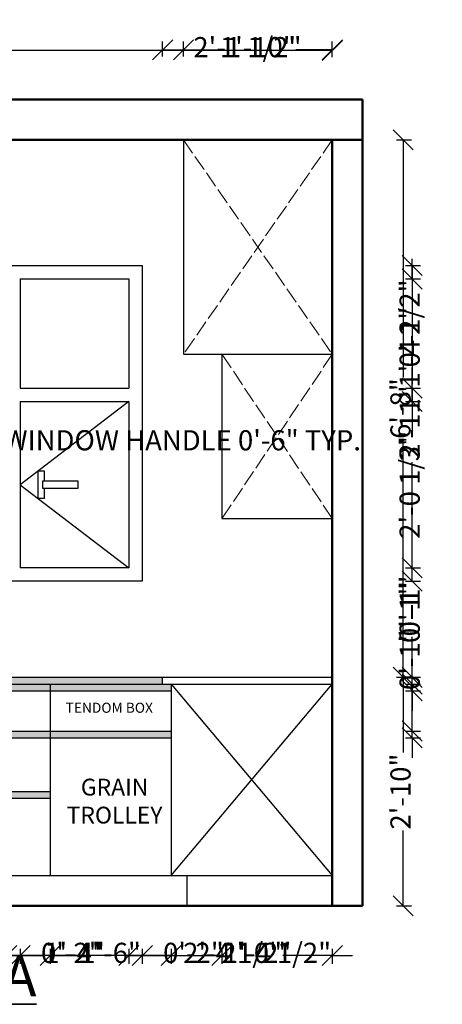
# Model space of a CAD drawing. Units: inches. Extents: x 2164 to 2316, y 625 to 771.
# Tile 2 of 2: x 2253 to 2316, y 625 to 771. Entities that reach past the tile are written whole.
import ezdxf

# ---------------------------------------------------------------- set-up
doc = ezdxf.new("R2010")
doc.units = ezdxf.units.IN
doc.linetypes.add('ACAD_ISO02W100', pattern=[15, 12, -3])
for name, color, linetype, lineweight in [('A-ANNO-DIMS', 2, 'Continuous', 18), ('A-ANNO-TEXT', 7, 'Continuous', 18), ('A-ANNO-TTLB', 7, 'Continuous', 35), ('A-FURN', 30, 'Continuous', 25), ('A-FURN-OPEN', 8, 'ACAD_ISO02W100', 13), ('A-FURN-PATT', 8, 'Continuous', 13), ('A-GLAZ', 4, 'Continuous', 25), ('A-WALL', 7, 'Continuous', 50)]:
    doc.layers.add(name, color=color, linetype=linetype, lineweight=lineweight)
doc.styles.get("Standard").update_dxf_attribs({"font": 'arial.ttf'})
doc.dimstyles.new('ISO-25', dxfattribs={"dimtxt": 3, "dimasz": 3, "dimexe": 1.25, "dimexo": 0.625, "dimtad": 0, "dimdec": 5, "dimlunit": 4, "dimtxsty": 'Standard', "dimblk": 'OBLIQUE', "dimcen": 2.5, "dimclrt": 1, "dimadec": 0, "dimazin": 0, "dimtfac": 1, "dimtdec": 5, "dimtmove": 0, "dimatfit": 3, "dimldrblk": 'OBLIQUE', "dimfxl": 1, "dimfxlon": 1, "dimfrac": 1, "dimarcsym": 0})

# ---------------------------------------------------------------- blocks, each defined once
blk = doc.blocks.new('_Oblique')
at = {"color": 0, "linetype": 'ByBlock', "lineweight": -2}
blk.add_line((-0.5, -0.5), (0.5, 0.5), dxfattribs=at)
blk = doc.blocks.new('*D4')
at = {"layer": 'A-ANNO-DIMS', "color": 0, "lineweight": -2, "transparency": 16777216}
for p, q in [((2180.45, 765.55), (2180.45, 767.8)), ((2180.45, 766.55), (2232.28, 766.55)), ((2299.95, 766.55), (2248.13, 766.55)), ((2299.95, 765.55), (2299.95, 767.8))]:
    blk.add_line(p, q, dxfattribs=at)
at = {"layer": 'Defpoints', "color": 0, "transparency": 16777216}
for p in [(2299.95, 766.55), (2180.45, 759.25), (2299.95, 759.25)]:
    blk.add_point(p, dxfattribs=at)
at = {"layer": 'A-ANNO-DIMS', "color": 0, "lineweight": -2, "transparency": 16777216, "xscale": 3, "yscale": 3, "zscale": 3, "rotation": 180}
blk.add_blockref('_Oblique', (2180.45, 766.55), dxfattribs=at)
at = {"layer": 'A-ANNO-DIMS', "color": 0, "lineweight": -2, "transparency": 16777216, "xscale": 3, "yscale": 3, "zscale": 3}
blk.add_blockref('_Oblique', (2299.95, 766.55), dxfattribs=at)
at = {"layer": 'A-ANNO-DIMS', "color": 0, "transparency": 16777216, "insert": (2240.2, 766.55), "char_height": 3, "attachment_point": 5}
blk.add_mtext('9\'-11{\\H1x;\\S1#2;}"', dxfattribs=at)
blk = doc.blocks.new('*D5')
at = {"layer": 'A-ANNO-DIMS', "color": 0, "lineweight": -2, "transparency": 16777216}
for p, q in [((2309.49, 673.25), (2311.74, 673.25)), ((2310.49, 673.25), (2310.49, 662.06)), ((2310.49, 639.25), (2310.49, 650.45)), ((2309.49, 639.25), (2311.74, 639.25))]:
    blk.add_line(p, q, dxfattribs=at)
at = {"layer": 'Defpoints', "color": 0, "transparency": 16777216}
for p in [(2299.95, 673.25), (2310.49, 673.25), (2299.95, 639.25)]:
    blk.add_point(p, dxfattribs=at)
at = {"layer": 'A-ANNO-DIMS', "color": 0, "lineweight": -2, "transparency": 16777216, "xscale": 3, "yscale": 3, "zscale": 3}
for p, rotation in [((2310.49, 673.25), 90), ((2310.49, 639.25), 270)]:
    blk.add_blockref('_Oblique', p, dxfattribs=dict(at, rotation=rotation))
at = {"layer": 'A-ANNO-DIMS', "color": 0, "transparency": 16777216, "insert": (2310.49, 656.25), "char_height": 3, "attachment_point": 5, "rotation": 90}
blk.add_mtext('2\'-10"', dxfattribs=at)
blk = doc.blocks.new('*D6')
at = {"layer": 'A-ANNO-DIMS', "color": 0, "lineweight": -2, "transparency": 16777216}
for p, q in [((2309.49, 753.25), (2311.74, 753.25)), ((2310.49, 753.25), (2310.49, 717.87)), ((2310.49, 673.25), (2310.49, 708.63)), ((2309.49, 673.25), (2311.74, 673.25))]:
    blk.add_line(p, q, dxfattribs=at)
at = {"layer": 'Defpoints', "color": 0, "transparency": 16777216}
for p in [(2299.95, 753.25), (2310.49, 753.25), (2299.95, 673.25)]:
    blk.add_point(p, dxfattribs=at)
at = {"layer": 'A-ANNO-DIMS', "color": 0, "lineweight": -2, "transparency": 16777216, "xscale": 3, "yscale": 3, "zscale": 3}
for p, rotation in [((2310.49, 753.25), 90), ((2310.49, 673.25), 270)]:
    blk.add_blockref('_Oblique', p, dxfattribs=dict(at, rotation=rotation))
at = {"layer": 'A-ANNO-DIMS', "color": 0, "transparency": 16777216, "insert": (2310.49, 713.25), "char_height": 3, "attachment_point": 5, "rotation": 90}
blk.add_mtext('6\'-8"', dxfattribs=at)
blk = doc.blocks.new('WIN-HANDLE')
blk.add_lwpolyline([(2239.92, 710.04), (2239.92, 709.04), (2240.92, 709.04), (2240.92, 710.54), (2245.92, 710.54), (2245.92, 711.54), (2240.92, 711.54), (2240.92, 713.04), (2239.92, 713.04), (2239.92, 711.04)], close=True)
blk.add_lwpolyline([(2240.92, 711.54), (2240.62, 711.54), (2240.62, 710.54), (2240.92, 710.54)])
blk = doc.blocks.new('*D8')
at = {"layer": 'A-ANNO-DIMS', "color": 0, "lineweight": -2, "transparency": 16777216}
for p, q in [((2239.92, 708.42), (2239.92, 706.89)), ((2239.92, 708.14), (2245.92, 708.14)), ((2245.92, 708.42), (2245.92, 706.89)), ((2245.92, 708.14), (2248.92, 708.14))]:
    blk.add_line(p, q, dxfattribs=at)
at = {"layer": 'Defpoints', "color": 0, "transparency": 16777216}
for p in [(2239.92, 709.04), (2245.92, 709.04), (2245.92, 708.14)]:
    blk.add_point(p, dxfattribs=at)
at = {"layer": 'A-ANNO-DIMS', "color": 0, "lineweight": -2, "transparency": 16777216, "xscale": 3, "yscale": 3, "zscale": 3, "rotation": 180}
blk.add_blockref('_Oblique', (2239.92, 708.14), dxfattribs=at)
at = {"layer": 'A-ANNO-DIMS', "color": 0, "lineweight": -2, "transparency": 16777216, "xscale": 3, "yscale": 3, "zscale": 3}
blk.add_blockref('_Oblique', (2245.92, 708.14), dxfattribs=at)
at = {"layer": 'A-ANNO-DIMS', "color": 1, "transparency": 16777216, "insert": (2277.61, 708.14), "char_height": 3, "attachment_point": 5}
blk.add_mtext('WINDOW HANDLE 0\'-6" TYP.', dxfattribs=at)
blk = doc.blocks.new('*D11')
at = {"layer": 'A-ANNO-DIMS', "color": 0, "lineweight": -2, "transparency": 16777216}
for p, q in [((2277.79, 765.65), (2277.79, 767.9)), ((2299.95, 765.65), (2299.95, 767.9)), ((2277.79, 766.65), (2283.23, 766.65)), ((2299.95, 766.65), (2294.51, 766.65))]:
    blk.add_line(p, q, dxfattribs=at)
at = {"layer": 'Defpoints', "color": 0, "transparency": 16777216}
for p in [(2299.95, 766.65), (2277.79, 753.25), (2299.95, 753.25)]:
    blk.add_point(p, dxfattribs=at)
at = {"layer": 'A-ANNO-DIMS', "color": 0, "lineweight": -2, "transparency": 16777216, "xscale": 3, "yscale": 3, "zscale": 3, "rotation": 180}
blk.add_blockref('_Oblique', (2277.79, 766.65), dxfattribs=at)
at = {"layer": 'A-ANNO-DIMS', "color": 0, "lineweight": -2, "transparency": 16777216, "xscale": 3, "yscale": 3, "zscale": 3}
blk.add_blockref('_Oblique', (2299.95, 766.65), dxfattribs=at)
at = {"layer": 'A-ANNO-DIMS', "color": 1, "transparency": 16777216, "insert": (2288.87, 766.65), "char_height": 3, "attachment_point": 5}
blk.add_mtext('1\'-10"', dxfattribs=at)
blk = doc.blocks.new('*D15')
at = {"layer": 'A-ANNO-DIMS', "color": 0, "lineweight": -2, "transparency": 16777216}
for p, q in [((2283.52, 631.85), (2280.52, 631.85)), ((2283.52, 632.85), (2283.52, 630.6)), ((2283.52, 631.85), (2283.77, 631.85)), ((2299.95, 631.85), (2299.7, 631.85)), ((2299.95, 632.85), (2299.95, 630.6)), ((2299.95, 631.85), (2302.95, 631.85))]:
    blk.add_line(p, q, dxfattribs=at)
at = {"layer": 'Defpoints', "color": 0, "transparency": 16777216}
for p in [(2283.52, 696.88), (2299.95, 696.88), (2299.95, 631.85)]:
    blk.add_point(p, dxfattribs=at)
at = {"layer": 'A-ANNO-DIMS', "color": 0, "lineweight": -2, "transparency": 16777216, "xscale": 3, "yscale": 3, "zscale": 3}
blk.add_blockref('_Oblique', (2283.52, 631.85), dxfattribs=at)
at = {"layer": 'A-ANNO-DIMS', "color": 0, "lineweight": -2, "transparency": 16777216, "xscale": 3, "yscale": 3, "zscale": 3, "rotation": 180}
blk.add_blockref('_Oblique', (2299.95, 631.85), dxfattribs=at)
at = {"layer": 'A-ANNO-DIMS', "color": 1, "transparency": 16777216, "insert": (2291.73, 631.85), "char_height": 3, "attachment_point": 5}
blk.add_mtext('1\'-4 1/2"', dxfattribs=at)
blk = doc.blocks.new('*D16')
at = {"layer": 'A-ANNO-DIMS', "color": 0, "lineweight": -2, "transparency": 16777216}
for p, q in [((2271.66, 632.85), (2271.66, 630.6)), ((2271.66, 631.85), (2277.68, 631.85)), ((2299.95, 631.85), (2293.94, 631.85)), ((2299.95, 632.85), (2299.95, 630.6))]:
    blk.add_line(p, q, dxfattribs=at)
at = {"layer": 'Defpoints', "color": 0, "transparency": 16777216}
for p in [(2299.95, 696.88), (2271.66, 687.55), (2299.95, 631.85)]:
    blk.add_point(p, dxfattribs=at)
at = {"layer": 'A-ANNO-DIMS', "color": 0, "lineweight": -2, "transparency": 16777216, "xscale": 3, "yscale": 3, "zscale": 3, "rotation": 180}
blk.add_blockref('_Oblique', (2271.66, 631.85), dxfattribs=at)
at = {"layer": 'A-ANNO-DIMS', "color": 0, "lineweight": -2, "transparency": 16777216, "xscale": 3, "yscale": 3, "zscale": 3}
blk.add_blockref('_Oblique', (2299.95, 631.85), dxfattribs=at)
at = {"layer": 'A-ANNO-DIMS', "color": 1, "transparency": 16777216, "insert": (2285.81, 631.85), "char_height": 3, "attachment_point": 5}
blk.add_mtext('2\'-4 1/2"', dxfattribs=at)
blk = doc.blocks.new('*D20')
at = {"layer": 'A-ANNO-DIMS', "color": 0, "lineweight": -2, "transparency": 16777216}
for p, q in [((2251.49, 632.85), (2251.49, 630.6)), ((2251.49, 631.85), (2253.49, 631.85)), ((2253.49, 632.85), (2253.49, 630.6)), ((2253.49, 631.85), (2256.49, 631.85))]:
    blk.add_line(p, q, dxfattribs=at)
at = {"layer": 'Defpoints', "color": 0, "transparency": 16777216}
for p in [(2251.49, 689.55), (2253.49, 689.55), (2253.49, 631.85)]:
    blk.add_point(p, dxfattribs=at)
at = {"layer": 'A-ANNO-DIMS', "color": 0, "lineweight": -2, "transparency": 16777216, "xscale": 3, "yscale": 3, "zscale": 3, "rotation": 180}
blk.add_blockref('_Oblique', (2251.49, 631.85), dxfattribs=at)
at = {"layer": 'A-ANNO-DIMS', "color": 0, "lineweight": -2, "transparency": 16777216, "xscale": 3, "yscale": 3, "zscale": 3}
blk.add_blockref('_Oblique', (2253.49, 631.85), dxfattribs=at)
at = {"layer": 'A-ANNO-DIMS', "color": 1, "transparency": 16777216, "insert": (2261.11, 631.85), "char_height": 3, "attachment_point": 5}
blk.add_mtext('0\'-2"', dxfattribs=at)
blk = doc.blocks.new('*D21')
at = {"layer": 'A-ANNO-DIMS', "color": 0, "lineweight": -2, "transparency": 16777216}
for p, q in [((2253.49, 632.85), (2253.49, 630.6)), ((2253.49, 631.85), (2257.11, 631.85)), ((2269.66, 631.85), (2266.05, 631.85)), ((2269.66, 632.85), (2269.66, 630.6))]:
    blk.add_line(p, q, dxfattribs=at)
at = {"layer": 'Defpoints', "color": 0, "transparency": 16777216}
for p in [(2253.49, 689.55), (2269.66, 689.55), (2269.66, 631.85)]:
    blk.add_point(p, dxfattribs=at)
at = {"layer": 'A-ANNO-DIMS', "color": 0, "lineweight": -2, "transparency": 16777216, "xscale": 3, "yscale": 3, "zscale": 3, "rotation": 180}
blk.add_blockref('_Oblique', (2253.49, 631.85), dxfattribs=at)
at = {"layer": 'A-ANNO-DIMS', "color": 0, "lineweight": -2, "transparency": 16777216, "xscale": 3, "yscale": 3, "zscale": 3}
blk.add_blockref('_Oblique', (2269.66, 631.85), dxfattribs=at)
at = {"layer": 'A-ANNO-DIMS', "color": 1, "transparency": 16777216, "insert": (2261.58, 631.85), "char_height": 3, "attachment_point": 5}
blk.add_mtext('1\'-4"', dxfattribs=at)
blk = doc.blocks.new('*D22')
at = {"layer": 'A-ANNO-DIMS', "color": 0, "lineweight": -2, "transparency": 16777216}
for p, q in [((2269.66, 632.85), (2269.66, 630.6)), ((2269.66, 631.85), (2271.66, 631.85)), ((2271.66, 632.85), (2271.66, 630.6)), ((2271.66, 631.85), (2274.66, 631.85))]:
    blk.add_line(p, q, dxfattribs=at)
at = {"layer": 'Defpoints', "color": 0, "transparency": 16777216}
for p in [(2269.66, 689.55), (2271.66, 687.55), (2271.66, 631.85)]:
    blk.add_point(p, dxfattribs=at)
at = {"layer": 'A-ANNO-DIMS', "color": 0, "lineweight": -2, "transparency": 16777216, "xscale": 3, "yscale": 3, "zscale": 3, "rotation": 180}
blk.add_blockref('_Oblique', (2269.66, 631.85), dxfattribs=at)
at = {"layer": 'A-ANNO-DIMS', "color": 0, "lineweight": -2, "transparency": 16777216, "xscale": 3, "yscale": 3, "zscale": 3}
blk.add_blockref('_Oblique', (2271.66, 631.85), dxfattribs=at)
at = {"layer": 'A-ANNO-DIMS', "color": 1, "transparency": 16777216, "insert": (2279.28, 631.85), "char_height": 3, "attachment_point": 5}
blk.add_mtext('0\'-2"', dxfattribs=at)
blk = doc.blocks.new('*D23')
at = {"layer": 'A-ANNO-DIMS', "color": 0, "lineweight": -2, "transparency": 16777216}
for p, q in [((2209.01, 632.85), (2209.01, 630.6)), ((2209.01, 631.85), (2232.23, 631.85)), ((2271.66, 631.85), (2248.44, 631.85)), ((2271.66, 632.85), (2271.66, 630.6))]:
    blk.add_line(p, q, dxfattribs=at)
at = {"layer": 'Defpoints', "color": 0, "transparency": 16777216}
for p in [(2209.01, 687.55), (2271.66, 687.55), (2271.66, 631.85)]:
    blk.add_point(p, dxfattribs=at)
at = {"layer": 'A-ANNO-DIMS', "color": 0, "lineweight": -2, "transparency": 16777216, "xscale": 3, "yscale": 3, "zscale": 3, "rotation": 180}
blk.add_blockref('_Oblique', (2209.01, 631.85), dxfattribs=at)
at = {"layer": 'A-ANNO-DIMS', "color": 0, "lineweight": -2, "transparency": 16777216, "xscale": 3, "yscale": 3, "zscale": 3}
blk.add_blockref('_Oblique', (2271.66, 631.85), dxfattribs=at)
at = {"layer": 'A-ANNO-DIMS', "color": 1, "transparency": 16777216, "insert": (2240.33, 631.85), "char_height": 3, "attachment_point": 5}
blk.add_mtext('5\'-2 1/2"', dxfattribs=at)
blk = doc.blocks.new('*D24')
at = {"layer": 'A-ANNO-DIMS', "color": 0, "lineweight": -2, "transparency": 16777216}
for p, q in [((2310.85, 734.54), (2313.1, 734.54)), ((2311.85, 734.54), (2311.85, 716.82)), ((2311.85, 687.55), (2311.85, 705.27)), ((2310.85, 687.55), (2313.1, 687.55))]:
    blk.add_line(p, q, dxfattribs=at)
at = {"layer": 'Defpoints', "color": 0, "transparency": 16777216}
for p in [(2271.66, 734.54), (2271.66, 687.55), (2311.85, 687.55)]:
    blk.add_point(p, dxfattribs=at)
at = {"layer": 'A-ANNO-DIMS', "color": 0, "lineweight": -2, "transparency": 16777216, "xscale": 3, "yscale": 3, "zscale": 3}
for p, rotation in [((2311.85, 734.54), 90), ((2311.85, 687.55), 270)]:
    blk.add_blockref('_Oblique', p, dxfattribs=dict(at, rotation=rotation))
at = {"layer": 'A-ANNO-DIMS', "color": 1, "transparency": 16777216, "insert": (2311.85, 711.05), "char_height": 3, "attachment_point": 5, "rotation": 90}
blk.add_mtext('3\'-11"', dxfattribs=at)
blk = doc.blocks.new('*D26')
at = {"layer": 'A-ANNO-DIMS', "color": 0, "lineweight": -2, "transparency": 16777216}
for p, q in [((2310.85, 714.29), (2313.1, 714.29)), ((2311.85, 714.29), (2311.85, 710.05)), ((2311.85, 689.55), (2311.85, 693.79)), ((2310.85, 689.55), (2313.1, 689.55))]:
    blk.add_line(p, q, dxfattribs=at)
at = {"layer": 'Defpoints', "color": 0, "transparency": 16777216}
for p in [(2269.66, 714.29), (2311.85, 714.29), (2269.66, 689.55)]:
    blk.add_point(p, dxfattribs=at)
at = {"layer": 'A-ANNO-DIMS', "color": 0, "lineweight": -2, "transparency": 16777216, "xscale": 3, "yscale": 3, "zscale": 3}
for p, rotation in [((2311.85, 714.29), 90), ((2311.85, 689.55), 270)]:
    blk.add_blockref('_Oblique', p, dxfattribs=dict(at, rotation=rotation))
at = {"layer": 'A-ANNO-DIMS', "color": 1, "transparency": 16777216, "insert": (2311.85, 701.92), "char_height": 3, "attachment_point": 5, "rotation": 90}
blk.add_mtext('2\'-0 1/2"', dxfattribs=at)
blk = doc.blocks.new('*D27')
at = {"layer": 'A-ANNO-DIMS', "color": 0, "lineweight": -2, "transparency": 16777216}
for p, q in [((2311.85, 716.29), (2311.85, 719.29)), ((2310.85, 716.29), (2313.1, 716.29)), ((2311.85, 714.29), (2311.85, 716.29)), ((2310.85, 714.29), (2313.1, 714.29))]:
    blk.add_line(p, q, dxfattribs=at)
at = {"layer": 'Defpoints', "color": 0, "transparency": 16777216}
for p in [(2269.66, 716.29), (2311.85, 716.29), (2269.66, 714.29)]:
    blk.add_point(p, dxfattribs=at)
at = {"layer": 'A-ANNO-DIMS', "color": 0, "lineweight": -2, "transparency": 16777216, "xscale": 3, "yscale": 3, "zscale": 3}
for p, rotation in [((2311.85, 716.29), 90), ((2311.85, 714.29), 270)]:
    blk.add_blockref('_Oblique', p, dxfattribs=dict(at, rotation=rotation))
at = {"layer": 'A-ANNO-DIMS', "color": 1, "transparency": 16777216, "insert": (2311.85, 723.9), "char_height": 3, "attachment_point": 5, "rotation": 90}
blk.add_mtext('0\'-2"', dxfattribs=at)
blk = doc.blocks.new('*D28')
at = {"layer": 'A-ANNO-DIMS', "color": 0, "lineweight": -2, "transparency": 16777216}
for p, q in [((2311.85, 732.54), (2311.85, 735.54)), ((2310.85, 732.54), (2313.1, 732.54)), ((2311.85, 732.54), (2311.85, 732.38)), ((2310.85, 716.29), (2313.1, 716.29)), ((2311.85, 716.29), (2311.85, 716.45)), ((2311.85, 716.29), (2311.85, 713.29))]:
    blk.add_line(p, q, dxfattribs=at)
at = {"layer": 'Defpoints', "color": 0, "transparency": 16777216}
for p in [(2269.66, 732.54), (2311.85, 732.54), (2269.66, 716.29)]:
    blk.add_point(p, dxfattribs=at)
at = {"layer": 'A-ANNO-DIMS', "color": 0, "lineweight": -2, "transparency": 16777216, "xscale": 3, "yscale": 3, "zscale": 3}
for p, rotation in [((2311.85, 732.54), 270), ((2311.85, 716.29), 90)]:
    blk.add_blockref('_Oblique', p, dxfattribs=dict(at, rotation=rotation))
at = {"layer": 'A-ANNO-DIMS', "color": 1, "transparency": 16777216, "insert": (2311.85, 724.42), "char_height": 3, "attachment_point": 5, "rotation": 90}
blk.add_mtext('1\'-4 1/2"', dxfattribs=at)
blk = doc.blocks.new('*D30')
at = {"layer": 'A-ANNO-DIMS', "color": 0, "lineweight": -2, "transparency": 16777216}
for p, q in [((2274.69, 765.65), (2274.69, 767.9)), ((2299.95, 765.65), (2299.95, 767.9)), ((2274.69, 766.65), (2279.19, 766.65)), ((2299.95, 766.65), (2295.45, 766.65))]:
    blk.add_line(p, q, dxfattribs=at)
at = {"layer": 'Defpoints', "color": 0, "transparency": 16777216}
for p in [(2299.95, 766.65), (2274.69, 673.25), (2299.95, 673.25)]:
    blk.add_point(p, dxfattribs=at)
at = {"layer": 'A-ANNO-DIMS', "color": 0, "lineweight": -2, "transparency": 16777216, "xscale": 3, "yscale": 3, "zscale": 3, "rotation": 180}
blk.add_blockref('_Oblique', (2274.69, 766.65), dxfattribs=at)
at = {"layer": 'A-ANNO-DIMS', "color": 0, "lineweight": -2, "transparency": 16777216, "xscale": 3, "yscale": 3, "zscale": 3}
blk.add_blockref('_Oblique', (2299.95, 766.65), dxfattribs=at)
at = {"layer": 'A-ANNO-DIMS', "color": 1, "transparency": 16777216, "insert": (2287.32, 766.65), "char_height": 3, "attachment_point": 5}
blk.add_mtext('2\'-1 1/2"', dxfattribs=at)
blk = doc.blocks.new('*D31')
at = {"layer": 'A-ANNO-DIMS', "color": 0, "lineweight": -2, "transparency": 16777216}
for p, q in [((2311.85, 672.25), (2311.85, 678.25)), ((2310.85, 672.25), (2313.1, 672.25)), ((2310.85, 671.25), (2313.1, 671.25)), ((2311.85, 671.25), (2311.85, 672.25)), ((2311.85, 671.25), (2311.85, 668.25))]:
    blk.add_line(p, q, dxfattribs=at)
at = {"layer": 'Defpoints', "color": 0, "transparency": 16777216}
for p in [(2275.95, 672.25), (2275.95, 671.25), (2311.85, 672.25)]:
    blk.add_point(p, dxfattribs=at)
at = {"layer": 'A-ANNO-DIMS', "color": 0, "lineweight": -2, "transparency": 16777216, "xscale": 3, "yscale": 3, "zscale": 3}
for p, rotation in [((2311.85, 672.25), 270), ((2311.85, 671.25), 90)]:
    blk.add_blockref('_Oblique', p, dxfattribs=dict(at, rotation=rotation))
at = {"layer": 'A-ANNO-DIMS', "color": 1, "transparency": 16777216, "insert": (2311.85, 682.87), "char_height": 3, "attachment_point": 5, "rotation": 90}
blk.add_mtext('0\'-1"', dxfattribs=at)
blk = doc.blocks.new('*D32')
at = {"layer": 'A-ANNO-DIMS', "color": 0, "lineweight": -2, "transparency": 16777216}
for p, q in [((2311.85, 673.25), (2311.85, 679.25)), ((2310.85, 673.25), (2313.1, 673.25)), ((2311.85, 672.25), (2311.85, 673.25)), ((2310.85, 672.25), (2313.1, 672.25)), ((2311.85, 672.25), (2311.85, 669.25))]:
    blk.add_line(p, q, dxfattribs=at)
at = {"layer": 'Defpoints', "color": 0, "transparency": 16777216}
for p in [(2274.69, 673.25), (2311.85, 673.25), (2274.69, 672.25)]:
    blk.add_point(p, dxfattribs=at)
at = {"layer": 'A-ANNO-DIMS', "color": 0, "lineweight": -2, "transparency": 16777216, "xscale": 3, "yscale": 3, "zscale": 3}
for p, rotation in [((2311.85, 673.25), 270), ((2311.85, 672.25), 90)]:
    blk.add_blockref('_Oblique', p, dxfattribs=dict(at, rotation=rotation))
at = {"layer": 'A-ANNO-DIMS', "color": 1, "transparency": 16777216, "insert": (2311.85, 683.87), "char_height": 3, "attachment_point": 5, "rotation": 90}
blk.add_mtext('0\'-1"', dxfattribs=at)
blk = doc.blocks.new('*D33')
at = {"layer": 'A-ANNO-DIMS', "color": 0, "lineweight": -2, "transparency": 16777216}
for p, q in [((2311.85, 665.25), (2311.85, 671.25)), ((2310.85, 665.25), (2313.1, 665.25)), ((2310.85, 664.25), (2313.1, 664.25)), ((2311.85, 664.25), (2311.85, 665.25)), ((2311.85, 664.25), (2311.85, 661.25))]:
    blk.add_line(p, q, dxfattribs=at)
at = {"layer": 'Defpoints', "color": 0, "transparency": 16777216}
for p in [(2275.95, 665.25), (2275.95, 664.25), (2311.85, 665.25)]:
    blk.add_point(p, dxfattribs=at)
at = {"layer": 'A-ANNO-DIMS', "color": 0, "lineweight": -2, "transparency": 16777216, "xscale": 3, "yscale": 3, "zscale": 3}
for p, rotation in [((2311.85, 665.25), 270), ((2311.85, 664.25), 90)]:
    blk.add_blockref('_Oblique', p, dxfattribs=dict(at, rotation=rotation))
at = {"layer": 'A-ANNO-DIMS', "color": 1, "transparency": 16777216, "insert": (2311.85, 675.87), "char_height": 3, "attachment_point": 5, "rotation": 90}
blk.add_mtext('0\'-1"', dxfattribs=at)
blk = doc.blocks.new('*D38')
at = {"layer": 'A-ANNO-DIMS', "color": 0, "lineweight": -2, "transparency": 16777216}
for p, q in [((2222.45, 632.85), (2222.45, 630.6)), ((2222.45, 631.85), (2230.9, 631.85)), ((2257.95, 631.85), (2249.5, 631.85)), ((2257.95, 632.85), (2257.95, 630.6))]:
    blk.add_line(p, q, dxfattribs=at)
at = {"layer": 'Defpoints', "color": 0, "transparency": 16777216}
for p in [(2222.45, 643.75), (2257.95, 643.75), (2257.95, 631.85)]:
    blk.add_point(p, dxfattribs=at)
at = {"layer": 'A-ANNO-DIMS', "color": 0, "lineweight": -2, "transparency": 16777216, "xscale": 3, "yscale": 3, "zscale": 3, "rotation": 180}
blk.add_blockref('_Oblique', (2222.45, 631.85), dxfattribs=at)
at = {"layer": 'A-ANNO-DIMS', "color": 0, "lineweight": -2, "transparency": 16777216, "xscale": 3, "yscale": 3, "zscale": 3}
blk.add_blockref('_Oblique', (2257.95, 631.85), dxfattribs=at)
at = {"layer": 'A-ANNO-DIMS', "color": 1, "transparency": 16777216, "insert": (2240.2, 631.85), "char_height": 3, "attachment_point": 5}
blk.add_mtext('2\'-11 1/2"', dxfattribs=at)
blk = doc.blocks.new('*D39')
at = {"layer": 'A-ANNO-DIMS', "color": 0, "lineweight": -2, "transparency": 16777216}
for p, q in [((2257.95, 632.85), (2257.95, 630.6)), ((2257.95, 631.85), (2262.48, 631.85)), ((2275.95, 631.85), (2271.42, 631.85)), ((2275.95, 632.85), (2275.95, 630.6))]:
    blk.add_line(p, q, dxfattribs=at)
at = {"layer": 'Defpoints', "color": 0, "transparency": 16777216}
for p in [(2257.95, 643.75), (2275.95, 643.75), (2275.95, 631.85)]:
    blk.add_point(p, dxfattribs=at)
at = {"layer": 'A-ANNO-DIMS', "color": 0, "lineweight": -2, "transparency": 16777216, "xscale": 3, "yscale": 3, "zscale": 3, "rotation": 180}
blk.add_blockref('_Oblique', (2257.95, 631.85), dxfattribs=at)
at = {"layer": 'A-ANNO-DIMS', "color": 0, "lineweight": -2, "transparency": 16777216, "xscale": 3, "yscale": 3, "zscale": 3}
blk.add_blockref('_Oblique', (2275.95, 631.85), dxfattribs=at)
at = {"layer": 'A-ANNO-DIMS', "color": 1, "transparency": 16777216, "insert": (2266.95, 631.85), "char_height": 3, "attachment_point": 5}
blk.add_mtext('1\'-6"', dxfattribs=at)
blk = doc.blocks.new('*D40')
at = {"layer": 'A-ANNO-DIMS', "color": 0, "lineweight": -2, "transparency": 16777216}
for p, q in [((2275.95, 632.85), (2275.95, 630.6)), ((2275.95, 631.85), (2283.32, 631.85)), ((2299.95, 631.85), (2292.59, 631.85)), ((2299.95, 632.85), (2299.95, 630.6))]:
    blk.add_line(p, q, dxfattribs=at)
at = {"layer": 'Defpoints', "color": 0, "transparency": 16777216}
for p in [(2275.95, 643.75), (2299.95, 643.75), (2299.95, 631.85)]:
    blk.add_point(p, dxfattribs=at)
at = {"layer": 'A-ANNO-DIMS', "color": 0, "lineweight": -2, "transparency": 16777216, "xscale": 3, "yscale": 3, "zscale": 3, "rotation": 180}
blk.add_blockref('_Oblique', (2275.95, 631.85), dxfattribs=at)
at = {"layer": 'A-ANNO-DIMS', "color": 0, "lineweight": -2, "transparency": 16777216, "xscale": 3, "yscale": 3, "zscale": 3}
blk.add_blockref('_Oblique', (2299.95, 631.85), dxfattribs=at)
at = {"layer": 'A-ANNO-DIMS', "color": 1, "transparency": 16777216, "insert": (2287.95, 631.85), "char_height": 3, "attachment_point": 5}
blk.add_mtext('2\'-0"', dxfattribs=at)

msp = doc.modelspace()

# ---------------------------------------------------------------- hatches: boundary and pattern name
at = {"layer": 'A-FURN-PATT'}
h = msp.add_hatch(color=256, dxfattribs=at)
h.dxf.hatch_style = 1
h.paths.add_polyline_path([(2274.687404, 673.253049), (2206.256774, 673.253049), (2206.256774, 672.253049), (2222.453229, 672.253049), (2257.953229, 672.253049), (2274.687404, 672.253049)])
h = msp.add_hatch(color=256, dxfattribs=at)
h.dxf.hatch_style = 1
h.paths.add_polyline_path([(2257.953229, 672.253049), (2222.453229, 672.253049), (2222.453229, 671.253049), (2257.953229, 671.253049)])
h.paths.add_polyline_path([(2257.953229, 665.253049), (2222.453229, 665.253049), (2222.453229, 664.253049), (2257.953229, 664.253049)])
h.paths.add_polyline_path([(2275.953229, 665.253049), (2257.953229, 665.253049), (2257.953229, 664.253049), (2275.953229, 664.253049)])
h.paths.add_polyline_path([(2257.953229, 656.253049), (2222.453229, 656.253049), (2222.453229, 655.253049), (2257.953229, 655.253049)])
h.paths.add_polyline_path([(2275.953229, 672.253049), (2257.953229, 672.253049), (2257.953229, 671.253049), (2275.953229, 671.253049)])
h.paths.add_polyline_path([(2215.731449, 672.253049), (2204.453229, 672.253049), (2204.453229, 671.253049), (2215.731449, 671.253049)])
h.paths.add_polyline_path([(2222.453229, 672.253049), (2215.731449, 672.253049), (2215.731449, 671.253049), (2222.453229, 671.253049)])

# ---------------------------------------------------------------- linework, layer by layer
at = {"layer": 'A-FURN'}
for p, q in [((2277.7869, 753.253049), (2277.7869, 721.327988)), ((2277.7869, 721.327988), (2299.953229, 721.327988)), ((2283.51521, 721.327988), (2283.51521, 696.882525)), ((2283.51521, 696.882525), (2299.953229, 696.882525)), ((2180.453229, 673.253049), (2299.953229, 673.253049)), ((2274.687404, 672.253049), (2274.687404, 673.253049)), ((2204.453229, 671.253049), (2275.953229, 671.253049)), ((2222.453229, 672.253049), (2257.953229, 672.253049)), ((2257.953229, 672.253049), (2257.953229, 643.753049)), ((2257.953229, 672.253049), (2275.953229, 672.253049)), ((2275.953229, 672.253049), (2275.953229, 643.753049)), ((2275.953229, 672.253049), (2299.953229, 643.753049)), ((2275.953229, 643.753049), (2299.953229, 672.253049)), ((2275.953229, 672.253049), (2299.953229, 672.253049)), ((2222.453229, 665.253049), (2275.953229, 665.253049)), ((2222.453229, 664.253049), (2275.953229, 664.253049)), ((2222.453229, 656.253049), (2257.953229, 656.253049)), ((2222.453229, 655.253049), (2257.953229, 655.253049)), ((2180.453229, 643.753049), (2299.953229, 643.753049)), ((2278.308987, 643.753049), (2278.308987, 639.253049))]:
    msp.add_line(p, q, dxfattribs=at)
at = {"layer": 'A-FURN-OPEN', "ltscale": 0.2}
for p, q in [((2277.7869, 753.253049), (2299.953229, 721.327988)), ((2299.953229, 753.253049), (2277.7869, 721.327988)), ((2299.953229, 721.327988), (2283.51521, 696.882525)), ((2299.953229, 696.882525), (2283.51521, 721.327988))]:
    msp.add_line(p, q, dxfattribs=at)
at = {"layer": 'A-GLAZ'}
for p, q in [((2253.49409, 732.541226), (2253.49409, 716.291226)), ((2253.49409, 732.541226), (2269.663741, 732.541226)), ((2269.663741, 732.541226), (2269.663741, 716.291226)), ((2253.49409, 716.291226), (2269.663741, 716.291226)), ((2253.49409, 714.291226), (2269.663741, 714.291226)), ((2253.49409, 714.291226), (2253.49409, 689.550561)), ((2269.663741, 714.291226), (2253.49409, 701.920894)), ((2269.663741, 714.291226), (2269.663741, 689.550561)), ((2253.49409, 701.920894), (2269.663741, 689.550561)), ((2269.663741, 689.550561), (2253.49409, 689.550561))]:
    msp.add_line(p, q, dxfattribs=at)
msp.add_lwpolyline([(2209.005798, 734.541226), (2271.663741, 734.541226), (2271.663741, 687.550561), (2209.005798, 687.550561)], close=True, dxfattribs=at)
at = {"layer": 'A-WALL'}
for p, q in [((2304.453229, 759.253049), (2175.953229, 759.253049)), ((2304.453229, 639.253049), (2304.453229, 759.253049)), ((2304.453229, 753.253049), (2175.953229, 753.253049)), ((2299.953229, 639.253049), (2299.953229, 753.253049)), ((2175.953229, 639.253049), (2304.453229, 639.253049))]:
    msp.add_line(p, q, dxfattribs=at)

# ---------------------------------------------------------------- block references
at = {"layer": 'A-GLAZ'}
msp.add_blockref('WIN-HANDLE', (16.193624, -9.117462), dxfattribs=at)

# ---------------------------------------------------------------- texts
at = {"layer": 'A-ANNO-TEXT', "attachment_point": 1}
for s, width, insert, char_height in [('TENDOM BOX', 15.70227385, (2260.250956, 669.469607), 1.5), ('\\pxqc;GRAIN\\PTROLLEY', 23.78004909, (2255.651212, 658.157515), 2.5)]:
    msp.add_mtext_dynamic_manual_height_columns(s, width=width, gutter_width=12.5, heights=[0], dxfattribs=dict(at, insert=insert, char_height=char_height))
at = {"layer": 'A-ANNO-TTLB', "insert": (2206.044532, 631.780545), "char_height": 6, "attachment_point": 1}
msp.add_mtext_dynamic_manual_height_columns('{\\LELEVATION A}', width=73.64161161, gutter_width=12.5, heights=[0], dxfattribs=at)

# ---------------------------------------------------------------- dimensions: what is measured, and where the dimension line sits
at = {"layer": 'A-ANNO-DIMS'}
for base, p1, p2, picture, middle in [((2299.953229, 766.653049), (2274.687404, 673.253049), (2299.953229, 673.253049), '*D30', (2287.320316, 766.653049)), ((2299.953229, 766.653049), (2277.7869, 753.253049), (2299.953229, 753.253049), '*D11', (2288.870064, 766.653049)), ((2299.953229, 631.853049), (2271.663741, 687.550561), (2299.953229, 696.882525), '*D16', (2285.808485, 631.853049)), ((2299.953229, 631.853049), (2283.51521, 696.882525), (2299.953229, 696.882525), '*D15', (2291.73422, 631.853049)), ((2253.49409, 631.853049), (2251.49409, 689.550561), (2253.49409, 689.550561), '*D20', (2261.106471, 631.853049)), ((2269.663741, 631.853049), (2253.49409, 689.550561), (2269.663741, 689.550561), '*D21', (2261.578916, 631.853049)), ((2271.663741, 631.853049), (2269.663741, 689.550561), (2271.663741, 687.550561), '*D22', (2279.276122, 631.853049)), ((2271.663741, 631.853049), (2209.005798, 687.550561), (2271.663741, 687.550561), '*D23', (2240.33477, 631.853049)), ((2257.953229, 631.853049), (2222.453229, 643.753049), (2257.953229, 643.753049), '*D38', (2240.203229, 631.853049)), ((2275.953229, 631.853049), (2257.953229, 643.753049), (2275.953229, 643.753049), '*D39', (2266.953229, 631.853049)), ((2299.953229, 631.853049), (2275.953229, 643.753049), (2299.953229, 643.753049), '*D40', (2287.953229, 631.853049))]:
    dim = msp.add_linear_dim(base=base, p1=p1, p2=p2, dimstyle='ISO-25', override={"dimdec": 1, "dimlfac": 1, "dimrnd": 0, "dimzin": 1, "dimdsep": 46, "dimlunit": 4, "dimfrac": 2}, dxfattribs=at)
    dim.commit()
    dim.dimension.update_dxf_attribs({"geometry": picture, "text_midpoint": middle})
dim = msp.add_linear_dim(base=(2299.953229, 766.546128), p1=(2180.453229, 759.253049), p2=(2299.953229, 759.253049), dimstyle='ISO-25', override={"dimclrd": 0, "dimclre": 0, "dimclrt": 0}, dxfattribs=at)
dim.commit()
dim.dimension.update_dxf_attribs({"geometry": '*D4', "text_midpoint": (2240.203229, 766.546128), "dimtype": 160})
for base, p1, p2, override, picture, middle in [((2310.494358, 753.253049), (2299.953229, 673.253049), (2299.953229, 753.253049), {"dimclrd": 0, "dimclre": 0, "dimclrt": 0}, '*D6', (2310.494358, 713.253049)), ((2311.853229, 687.550561), (2271.663741, 734.541226), (2271.663741, 687.550561), {"dimdec": 1, "dimlfac": 1, "dimrnd": 0, "dimzin": 1, "dimdsep": 46, "dimlunit": 4, "dimfrac": 2}, '*D24', (2311.853229, 711.045893)), ((2311.853229, 732.541226), (2269.663741, 716.291226), (2269.663741, 732.541226), {"dimdec": 1, "dimlfac": 1, "dimrnd": 0, "dimzin": 1, "dimdsep": 46, "dimlunit": 4, "dimfrac": 2}, '*D28', (2311.853229, 724.416226)), ((2311.853229, 716.291226), (2269.663741, 714.291226), (2269.663741, 716.291226), {"dimdec": 1, "dimlfac": 1, "dimrnd": 0, "dimzin": 1, "dimdsep": 46, "dimlunit": 4, "dimfrac": 2}, '*D27', (2311.853229, 723.903607)), ((2311.853229, 714.291226), (2269.663741, 689.550561), (2269.663741, 714.291226), {"dimdec": 1, "dimlfac": 1, "dimrnd": 0, "dimzin": 1, "dimdsep": 46, "dimlunit": 4, "dimfrac": 2}, '*D26', (2311.853229, 701.920893)), ((2311.853229, 673.253049), (2274.687404, 672.253049), (2274.687404, 673.253049), {"dimdec": 1, "dimlfac": 1, "dimrnd": 0, "dimzin": 1, "dimdsep": 46, "dimlunit": 4, "dimfrac": 2}, '*D32', (2311.853229, 683.86543)), ((2311.853229, 672.253049), (2275.953229, 671.253049), (2275.953229, 672.253049), {"dimdec": 1, "dimlfac": 1, "dimrnd": 0, "dimzin": 1, "dimdsep": 46, "dimlunit": 4, "dimfrac": 2}, '*D31', (2311.853229, 682.86543)), ((2311.853229, 665.253049), (2275.953229, 664.253049), (2275.953229, 665.253049), {"dimdec": 1, "dimlfac": 1, "dimrnd": 0, "dimzin": 1, "dimdsep": 46, "dimlunit": 4, "dimfrac": 2}, '*D33', (2311.853229, 675.86543)), ((2310.494358, 673.253049), (2299.953229, 639.253049), (2299.953229, 673.253049), {"dimclrd": 0, "dimclre": 0, "dimclrt": 0}, '*D5', (2310.494358, 656.253049))]:
    dim = msp.add_linear_dim(base=base, p1=p1, p2=p2, angle=90, dimstyle='ISO-25', override=override, dxfattribs=at)
    dim.commit()
    dim.dimension.update_dxf_attribs({"geometry": picture, "text_midpoint": middle})
dim = msp.add_linear_dim(base=(2245.920421, 708.142709), p1=(2239.920421, 709.042709), p2=(2245.920421, 709.042709), text='WINDOW HANDLE <> TYP.', dimstyle='ISO-25', override={"dimdec": 1, "dimlfac": 1, "dimrnd": 0, "dimzin": 1, "dimdsep": 46, "dimlunit": 4, "dimfrac": 2}, dxfattribs=at)
dim.commit()
dim.dimension.update_dxf_attribs({"geometry": '*D8', "text_midpoint": (2277.609541, 708.142709)})

doc.saveas('drawing.dxf')
